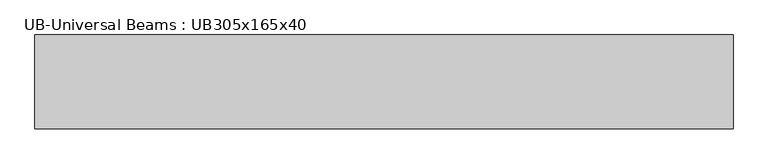
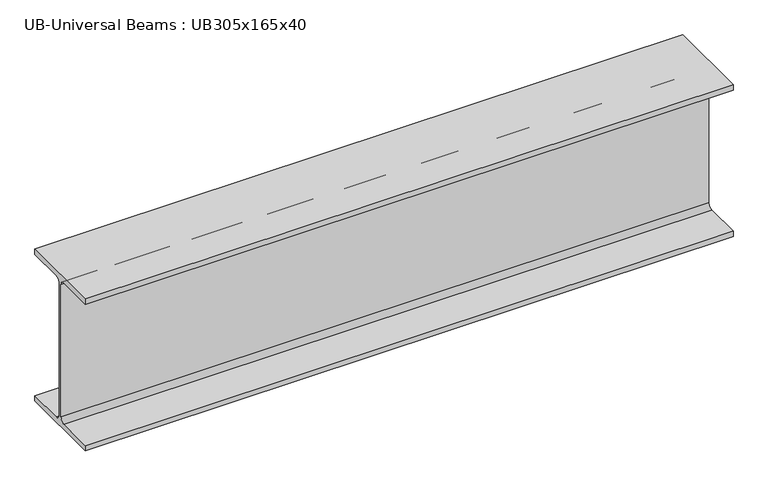
"""IFC4 building model written with IfcOpenShell, lengths in millimetres: beam geometry, UB-Universal Beams : UB305x165x40."""

from ifc_helpers import new_model, si_unit, point, frame, frame_2d, origin, place, context, project, spatial, polyline, circle_curve, trimmed, segment, composite_curve, outline, extrude, source, transform, mapped, element, save


def ub_universal_beams_ub305x165x40_83ed4f69(model_context):
    return source(origin(), model_context, "Body", "SweptSolid", [
        extrude(outline(composite_curve([segment(polyline([(82.5, -141.5), (82.5, -151.7), (-82.5, -151.7), (-82.5, -141.5), (-11.9, -141.5)]), True, "CONTINUOUS"), segment(trimmed(circle_curve(frame_2d((-11.9, -132.6)), 8.9), [point((-11.9, -141.5))], [point((-3.0, -132.6))], True, "CARTESIAN"), True, "CONTINUOUS"), segment(polyline([(-3.0, -132.6), (-3.0, 132.6)]), True, "CONTINUOUS"), segment(trimmed(circle_curve(frame_2d((-11.9, 132.6)), 8.9), [point((-3.0, 132.6))], [point((-11.9, 141.5))], True, "CARTESIAN"), True, "CONTINUOUS"), segment(polyline([(-11.9, 141.5), (-82.5, 141.5), (-82.5, 151.7), (82.5, 151.7), (82.5, 141.5), (11.9, 141.5)]), True, "CONTINUOUS"), segment(trimmed(circle_curve(frame_2d((11.9, 132.6)), 8.9), [point((11.9, 141.5))], [point((3.0, 132.6))], True, "CARTESIAN"), True, "CONTINUOUS"), segment(polyline([(3.0, 132.6), (3.0, -132.6)]), True, "CONTINUOUS"), segment(trimmed(circle_curve(frame_2d((11.9, -132.6)), 8.9), [point((3.0, -132.6))], [point((11.9, -141.5))], True, "CARTESIAN"), True, "CONTINUOUS"), segment(polyline([(11.9, -141.5), (82.5, -141.5)]), True, "CONTINUOUS")], self_intersect=False)), frame((-600.05, 0.0, 0.0), z_axis=(1.0, 0.0, 0.0), x_axis=(0.0, 1.0, 0.0)), (0.0, 0.0, 1.0), 1225.9),
    ])


if __name__ == "__main__":
    model = new_model("IFC4")
    model_context = context("Model", 3, world=origin())
    ifc_project = project(units=[si_unit("LENGTHUNIT", "METRE", prefix="MILLI")], contexts=[model_context])
    site = spatial("IfcSite", under=ifc_project)
    building = spatial("IfcBuilding", under=site)
    placement = place(None, origin())
    ub_universal_beams_ub305x165x40_shape = ub_universal_beams_ub305x165x40_83ed4f69(model_context)
    element("IfcBeam", 1, ObjectType="UB-Universal Beams : UB305x165x40", at=placement, inside=building, context=model_context, shape_type="MappedRepresentation", body=[
        mapped(ub_universal_beams_ub305x165x40_shape, transform((0.0, 0.0, 0.0), x_axis=(1.0, 0.0, 0.0), y_axis=(0.0, 1.0, 0.0), z_axis=(0.0, 0.0, 1.0))),
    ])
    save(model, "model.ifc")

# Revit data of these elements
# Type "UB-Universal Beams : UB305x165x40"
#   Section Name Key = "UB305X165X40"
#   Width = 16.5 cm
#   Web Thickness = 0.6 cm
#   Web Fillet = 0.89 cm
#   Warping Constant = 164000.0 cm⁶
#   Torsional Moment of Inertia = 14.70 cm⁴
#   Section Area = 51.3 cm²
#   Plastic Modulus weak axis = 142.0 cm³
#   Plastic Modulus strong axis = 623.0 cm³
#   Nominal Weight = 40.2999 kgf/m
#   Moment of Inertia weak axis = 764.00 cm⁴
#   Moment of Inertia strong axis = 8503.00 cm⁴
#   Height = 30.34 cm
#   Flange Thickness = 1.02 cm
#   Elastic Modulus weak axis = 92.6 cm³
#   Elastic Modulus strong axis = 560.0 cm³
#   Centroid Vertical = 15.17 cm
#   Centroid Horizontal = 8.25 cm
#   Bolt Spacing = 9.0 cm
#   Length [instance default] = 1500 mm
#   Structural Material [instance default] = Metal - Steel 43-275
#   Type Comments = ""
#   Assembly Code = ""
# Element 1 (IfcBeam, "UB-Universal Beams : UB305x165x40")
#   Materials on its faces: "Metal - Steel 43-275"
# Materials
#   "Metal - Steel 43-275": class "Metal", colour RGB 247 247 247, transparency 0, Cost = 0
